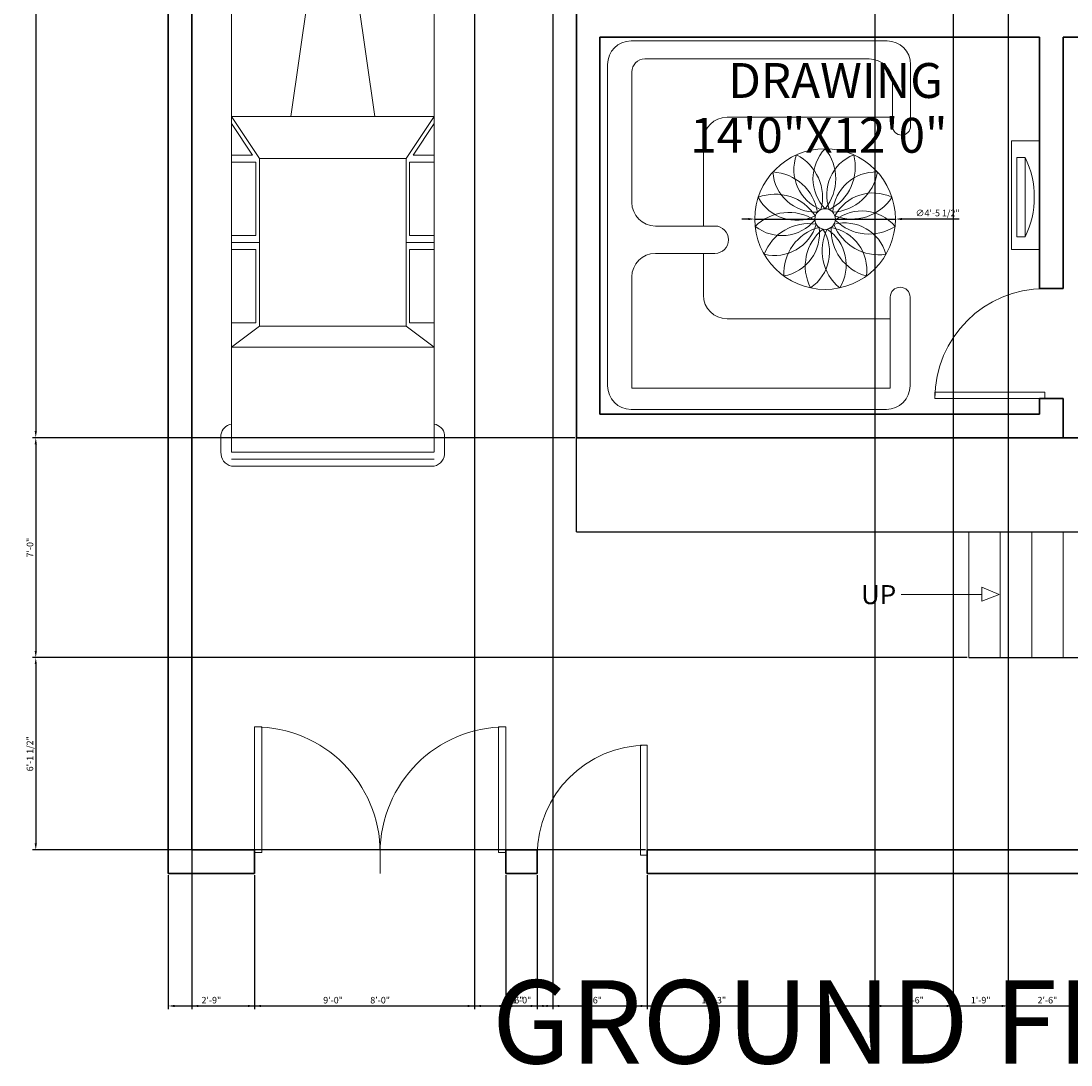
# Model space of a CAD drawing. Units: inches. Extents: x 3412 to 4225, y 13529 to 14581.
# Tile 1 of 7: x 3412 to 3813, y 13529 to 13928. Entities that reach past the tile are written whole.
import ezdxf

# ---------------------------------------------------------------- set-up
doc = ezdxf.new("R2010")
doc.units = ezdxf.units.IN
for name, color, linetype, lineweight in [('A-ANNO-DIMS', 2, 'Continuous', 13), ('A-ANNO-SYMB', 2, 'Continuous', 13), ('A-ANNO-TEXT', 7, 'Continuous', 18), ('A-ANNO-TITL', 7, 'Continuous', 35), ('A-AREA-IDEN', 7, 'Continuous', 18), ('A-DOOR', 4, 'Continuous', 18), ('A-FLOR', 7, 'Continuous', 25), ('A-FLOR-STRS', 3, 'Continuous', 18), ('A-FURN', 8, 'Continuous', 18), ('A-WALL', 7, 'Continuous', 35), ('C-PKNG-VEHI', 8, 'Continuous', 13), ('C-SITE-GATE', 4, 'Continuous', 18), ('C-SITE-WALL', 7, 'Continuous', 35)]:
    doc.layers.add(name, color=color, linetype=linetype, lineweight=lineweight)
doc.styles.get("Standard").update_dxf_attribs({"font": 'arial.ttf'})
doc.dimstyles.new('ISO-25', dxfattribs={"dimtxt": 2.5, "dimasz": 2.5, "dimexe": 1.25, "dimexo": 0.625, "dimtad": 1, "dimdec": 0, "dimlunit": 3, "dimtxsty": 'Standard', "dimcen": 2.5, "dimadec": 0, "dimazin": 0, "dimtfac": 1, "dimtdec": 0, "dimtmove": 0, "dimatfit": 3, "dimfxl": 1, "dimarcsym": 0})

# ---------------------------------------------------------------- blocks, each defined once
blk = doc.blocks.new('*U3')
for p, q in [((0, 0), (0, -5)), ((30, 0), (30, -5))]:
    blk.add_line(p, q)
blk.add_lwpolyline([(0, 0), (0, 30), (1.75, 30), (1.75, 0)], close=True)
blk.add_arc((0, 0), 30, 0, 90)
blk = doc.blocks.new('*U8')
for centre, radius, start, end in [((12.16, 0), 16.5, 135.9523, 224.0477), ((-13.92, 0), 18.27, 321.0981, 38.9019)]:
    blk.add_arc(centre, radius, start, end)
blk = doc.blocks.new('*U9')
at = {"layer": 'A-FURN', "color": 0, "linetype": 'ByBlock', "lineweight": -2, "transparency": 16777216}
for p, rotation in [((3712.86, 13866.4), 24.00000000000002), ((3725.39, 13866.64), 336.0000000000001), ((3707.75, 13862.54), 48.00000000000004), ((3730.64, 13862.98), 312), ((3704.65, 13856.93), 72.00000000000001), ((3733.95, 13857.49), 288), ((3704.11, 13850.55), 96.00000000000003), ((3734.74, 13851.14), 264.0000000000001), ((3706.2, 13844.5), 120), ((3710.58, 13839.82), 144), ((3728.68, 13840.17), 216), ((3732.88, 13845.01), 240), ((3716.48, 13837.33), 168), ((3722.88, 13837.45), 192)]:
    blk.add_blockref('*U8', p, dxfattribs=dict(at, rotation=rotation))
blk.add_blockref('*U8', (3719.1, 13867.85), dxfattribs=at)
blk = doc.blocks.new('*U20')
for p, q in [((5.44, 42.31), (12.12, 42.31)), ((189.69, 42.31), (183.01, 42.31)), ((0.1, -0.41), (0.1, 38.35)), ((2.77, -0.41), (2.77, 38.31)), ((5.44, -0.41), (5.44, 38.24)), ((5.45, 38.31), (16.12, 38.31)), ((16.12, 38.31), (180.34, 38.31)), ((61.52, -0.41), (61.52, 38.31)), ((61.52, 38.31), (77.54, 27.62)), ((64.19, 38.31), (76.2, 30.29)), ((76.2, 30.29), (76.2, 38.31)), ((78.87, 38.31), (78.87, 28.96)), ((106.91, 28.96), (106.91, 38.31)), ((109.58, 27.62), (109.58, 38.31)), ((112.25, 38.31), (112.25, 28.96)), ((140.29, 28.96), (140.29, 38.31)), ((141.62, 27.62), (149.64, 38.31)), ((149.64, -0.41), (149.64, 38.31)), ((189.69, 38.31), (179.01, 38.31)), ((189.69, -0.41), (189.69, 38.24)), ((192.36, -0.41), (192.36, 38.31)), ((195.03, -0.41), (195.03, 38.35)), ((78.87, 28.96), (106.91, 28.96)), ((112.25, 28.96), (140.29, 28.96)), ((77.54, 27.62), (141.62, 27.62)), ((77.54, -0.41), (77.54, 27.62)), ((141.62, -0.41), (141.62, 27.62)), ((5.44, 7.6), (61.52, 15.61)), ((0.1, -0.42), (0.1, -39.18)), ((2.77, -0.41), (2.77, -39.13)), ((5.44, -0.42), (5.44, -39.07)), ((61.52, -0.41), (61.52, -39.13)), ((77.54, -0.41), (77.54, -28.45)), ((141.62, -0.41), (141.62, -28.45)), ((149.64, -0.41), (149.64, -39.13)), ((189.69, -0.42), (189.69, -39.07)), ((192.36, -0.41), (192.36, -39.13)), ((195.03, -0.42), (195.03, -39.18)), ((5.44, -8.42), (61.52, -16.43)), ((61.52, -39.13), (77.54, -28.45)), ((64.19, -39.13), (76.2, -31.12)), ((76.2, -31.12), (76.2, -39.13)), ((77.54, -28.45), (141.62, -28.45)), ((78.87, -39.13), (78.87, -29.79)), ((78.87, -29.79), (106.91, -29.79)), ((106.91, -29.79), (106.91, -39.13)), ((109.58, -28.45), (109.58, -39.13)), ((112.25, -29.79), (140.29, -29.79)), ((112.25, -39.13), (112.25, -29.79)), ((140.29, -29.79), (140.29, -39.13)), ((141.62, -28.45), (149.64, -39.13)), ((5.45, -39.13), (16.12, -39.13)), ((16.12, -39.13), (180.34, -39.13)), ((189.69, -39.13), (179.01, -39.13)), ((5.44, -43.14), (12.12, -43.14)), ((189.69, -43.14), (183.01, -43.14))]:
    blk.add_line(p, q)
for centre, radius, start, end in [((5.06, 37.26), 5.06, 85.6455, 168.0943), ((11.45, 37.64), 4.72, 8.1301, 81.87), ((183.68, 37.64), 4.72, 98.13, 171.8699), ((190.07, 37.26), 5.06, 11.9057, 94.3545), ((5.06, -38.09), 5.06, 191.9057, 274.3545), ((11.45, -38.46), 4.72, 278.13, 351.8699), ((183.68, -38.46), 4.72, 188.1301, 261.87), ((190.07, -38.09), 5.06, 265.6455, 348.0943)]:
    blk.add_arc(centre, radius, start, end)
blk = doc.blocks.new('ARROW-ENTRY-STEP')
for p, q in [((30.86, 5.34), (37.49, 2.66)), ((30.86, 0), (30.86, 5.34)), ((0, 2.66), (30.86, 2.66)), ((37.49, 2.66), (30.86, 0))]:
    blk.add_line(p, q)
blk = doc.blocks.new('ENTRY-STEP-FLIGHT')
for p, q in [((0, 48), (0, 0)), ((12, 48), (12, 0)), ((24, 48), (24, 0)), ((36, 48), (36, 0))]:
    blk.add_line(p, q)
blk = doc.blocks.new('*D61')
at = {"layer": 'A-ANNO-DIMS', "color": 0, "lineweight": -2, "transparency": 16777216}
for p, q in [((3477.36, 14408.81), (3477.36, 13550.58)), ((3585.36, 14408.81), (3585.36, 13550.58)), ((3479.86, 13551.83), (3582.86, 13551.83))]:
    blk.add_line(p, q, dxfattribs=at)
at = {"layer": 'A-ANNO-DIMS', "color": 0, "transparency": 16777216}
for points in [[(3479.86, 13552.25), (3479.86, 13551.42), (3477.36, 13551.83)], [(3582.86, 13552.25), (3582.86, 13551.42), (3585.36, 13551.83)]]:
    blk.add_solid(points, dxfattribs=at)
at = {"layer": 'Defpoints', "color": 0, "transparency": 16777216}
for p in [(3477.36, 14409.43), (3585.36, 14409.43), (3585.36, 13551.83)]:
    blk.add_point(p, dxfattribs=at)
at = {"layer": 'A-ANNO-DIMS', "color": 0, "transparency": 16777216, "insert": (3531.36, 13553.73), "char_height": 2.5, "attachment_point": 5}
blk.add_mtext('9\'-0"', dxfattribs=at)
blk = doc.blocks.new('*D62')
at = {"layer": 'A-ANNO-DIMS', "color": 0, "lineweight": -2, "transparency": 16777216}
for p, q in [((3585.36, 14408.81), (3585.36, 13550.58)), ((3615.36, 14408.81), (3615.36, 13550.58)), ((3587.86, 13551.83), (3612.86, 13551.83))]:
    blk.add_line(p, q, dxfattribs=at)
at = {"layer": 'A-ANNO-DIMS', "color": 0, "transparency": 16777216}
for points in [[(3587.86, 13552.25), (3587.86, 13551.42), (3585.36, 13551.83)], [(3612.86, 13552.25), (3612.86, 13551.42), (3615.36, 13551.83)]]:
    blk.add_solid(points, dxfattribs=at)
at = {"layer": 'Defpoints', "color": 0, "transparency": 16777216}
for p in [(3585.36, 14409.43), (3615.36, 14409.43), (3615.36, 13551.83)]:
    blk.add_point(p, dxfattribs=at)
at = {"layer": 'A-ANNO-DIMS', "color": 0, "transparency": 16777216, "insert": (3600.36, 13553.73), "char_height": 2.5, "attachment_point": 5}
blk.add_mtext('2\'-6"', dxfattribs=at)
blk = doc.blocks.new('*D63')
at = {"layer": 'A-ANNO-DIMS', "color": 0, "lineweight": -2, "transparency": 16777216}
for p, q in [((3615.36, 14408.81), (3615.36, 13550.58)), ((3738.36, 14408.81), (3738.36, 13550.58)), ((3617.86, 13551.83), (3735.86, 13551.83))]:
    blk.add_line(p, q, dxfattribs=at)
at = {"layer": 'A-ANNO-DIMS', "color": 0, "transparency": 16777216}
for points in [[(3617.86, 13552.25), (3617.86, 13551.42), (3615.36, 13551.83)], [(3735.86, 13552.25), (3735.86, 13551.42), (3738.36, 13551.83)]]:
    blk.add_solid(points, dxfattribs=at)
at = {"layer": 'Defpoints', "color": 0, "transparency": 16777216}
for p in [(3615.36, 14409.43), (3738.36, 14409.43), (3738.36, 13551.83)]:
    blk.add_point(p, dxfattribs=at)
at = {"layer": 'A-ANNO-DIMS', "color": 0, "transparency": 16777216, "insert": (3676.86, 13553.73), "char_height": 2.5, "attachment_point": 5}
blk.add_mtext('10\'-3"', dxfattribs=at)
blk = doc.blocks.new('*D64')
at = {"layer": 'A-ANNO-DIMS', "color": 0, "lineweight": -2, "transparency": 16777216}
for p, q in [((3738.36, 14408.81), (3738.36, 13550.58)), ((3768.36, 14408.81), (3768.36, 13550.58)), ((3740.86, 13551.83), (3765.86, 13551.83))]:
    blk.add_line(p, q, dxfattribs=at)
at = {"layer": 'A-ANNO-DIMS', "color": 0, "transparency": 16777216}
for points in [[(3740.86, 13552.25), (3740.86, 13551.42), (3738.36, 13551.83)], [(3765.86, 13552.25), (3765.86, 13551.42), (3768.36, 13551.83)]]:
    blk.add_solid(points, dxfattribs=at)
at = {"layer": 'Defpoints', "color": 0, "transparency": 16777216}
for p in [(3738.36, 14409.43), (3768.36, 14409.43), (3768.36, 13551.83)]:
    blk.add_point(p, dxfattribs=at)
at = {"layer": 'A-ANNO-DIMS', "color": 0, "transparency": 16777216, "insert": (3753.36, 13553.73), "char_height": 2.5, "attachment_point": 5}
blk.add_mtext('2\'-6"', dxfattribs=at)
blk = doc.blocks.new('*D65')
at = {"layer": 'A-ANNO-DIMS', "color": 0, "lineweight": -2, "transparency": 16777216}
for p, q in [((3768.36, 14408.81), (3768.36, 13550.58)), ((3789.36, 14408.81), (3789.36, 13550.58)), ((3770.86, 13551.83), (3786.86, 13551.83))]:
    blk.add_line(p, q, dxfattribs=at)
at = {"layer": 'A-ANNO-DIMS', "color": 0, "transparency": 16777216}
for points in [[(3770.86, 13552.25), (3770.86, 13551.42), (3768.36, 13551.83)], [(3786.86, 13552.25), (3786.86, 13551.42), (3789.36, 13551.83)]]:
    blk.add_solid(points, dxfattribs=at)
at = {"layer": 'Defpoints', "color": 0, "transparency": 16777216}
for p in [(3768.36, 14409.43), (3789.36, 14409.43), (3789.36, 13551.83)]:
    blk.add_point(p, dxfattribs=at)
at = {"layer": 'A-ANNO-DIMS', "color": 0, "transparency": 16777216, "insert": (3778.86, 13553.73), "char_height": 2.5, "attachment_point": 5}
blk.add_mtext('1\'-9"', dxfattribs=at)
blk = doc.blocks.new('*D66')
at = {"layer": 'A-ANNO-DIMS', "color": 0, "lineweight": -2, "transparency": 16777216}
for p, q in [((3789.36, 14408.81), (3789.36, 13550.58)), ((3819.36, 14408.81), (3819.36, 13550.58)), ((3791.86, 13551.83), (3816.86, 13551.83))]:
    blk.add_line(p, q, dxfattribs=at)
at = {"layer": 'A-ANNO-DIMS', "color": 0, "transparency": 16777216}
for points in [[(3791.86, 13552.25), (3791.86, 13551.42), (3789.36, 13551.83)], [(3816.86, 13552.25), (3816.86, 13551.42), (3819.36, 13551.83)]]:
    blk.add_solid(points, dxfattribs=at)
at = {"layer": 'Defpoints', "color": 0, "transparency": 16777216}
for p in [(3789.36, 14409.43), (3819.36, 14409.43), (3819.36, 13551.83)]:
    blk.add_point(p, dxfattribs=at)
at = {"layer": 'A-ANNO-DIMS', "color": 0, "transparency": 16777216, "insert": (3804.36, 13553.73), "char_height": 2.5, "attachment_point": 5}
blk.add_mtext('2\'-6"', dxfattribs=at)
blk = doc.blocks.new('*D74')
at = {"layer": 'A-ANNO-DIMS', "color": 0, "lineweight": -2, "transparency": 16777216}
for p, q in [((3593.73, 14199.43), (3416.51, 14199.43)), ((3417.76, 14196.93), (3417.76, 13771.43)), ((3623.73, 13768.93), (3416.51, 13768.93))]:
    blk.add_line(p, q, dxfattribs=at)
at = {"layer": 'A-ANNO-DIMS', "color": 0, "transparency": 16777216}
for points in [[(3417.34, 14196.93), (3418.17, 14196.93), (3417.76, 14199.43)], [(3417.34, 13771.43), (3418.17, 13771.43), (3417.76, 13768.93)]]:
    blk.add_solid(points, dxfattribs=at)
at = {"layer": 'Defpoints', "color": 0, "transparency": 16777216}
for p in [(3594.36, 14199.43), (3417.76, 13768.93), (3624.36, 13768.93)]:
    blk.add_point(p, dxfattribs=at)
at = {"layer": 'A-ANNO-DIMS', "color": 0, "transparency": 16777216, "insert": (3415.84, 13984.18), "char_height": 2.5, "attachment_point": 5, "rotation": 90}
blk.add_mtext('35\'-10 1/2"', dxfattribs=at)
blk = doc.blocks.new('*D75')
at = {"layer": 'A-ANNO-DIMS', "color": 0, "lineweight": -2, "transparency": 16777216}
for p, q in [((3623.73, 13768.93), (3416.51, 13768.93)), ((3417.76, 13766.43), (3417.76, 13687.43)), ((3773.73, 13684.93), (3416.51, 13684.93))]:
    blk.add_line(p, q, dxfattribs=at)
at = {"layer": 'A-ANNO-DIMS', "color": 0, "transparency": 16777216}
for points in [[(3417.34, 13766.43), (3418.17, 13766.43), (3417.76, 13768.93)], [(3417.34, 13687.43), (3418.17, 13687.43), (3417.76, 13684.93)]]:
    blk.add_solid(points, dxfattribs=at)
at = {"layer": 'Defpoints', "color": 0, "transparency": 16777216}
for p in [(3624.36, 13768.93), (3417.76, 13684.93), (3774.36, 13684.93)]:
    blk.add_point(p, dxfattribs=at)
at = {"layer": 'A-ANNO-DIMS', "color": 0, "transparency": 16777216, "insert": (3415.86, 13726.93), "char_height": 2.5, "attachment_point": 5, "rotation": 90}
blk.add_mtext('7\'-0"', dxfattribs=at)
blk = doc.blocks.new('*D76')
at = {"layer": 'A-ANNO-DIMS', "color": 0, "lineweight": -2, "transparency": 16777216}
for p, q in [((3773.73, 13684.93), (3416.51, 13684.93)), ((3417.76, 13682.43), (3417.76, 13613.93)), ((3650.73, 13611.43), (3416.51, 13611.43))]:
    blk.add_line(p, q, dxfattribs=at)
at = {"layer": 'A-ANNO-DIMS', "color": 0, "transparency": 16777216}
for points in [[(3417.34, 13682.43), (3418.17, 13682.43), (3417.76, 13684.93)], [(3417.34, 13613.93), (3418.17, 13613.93), (3417.76, 13611.43)]]:
    blk.add_solid(points, dxfattribs=at)
at = {"layer": 'Defpoints', "color": 0, "transparency": 16777216}
for p in [(3774.36, 13684.93), (3417.76, 13611.43), (3651.36, 13611.43)]:
    blk.add_point(p, dxfattribs=at)
at = {"layer": 'A-ANNO-DIMS', "color": 0, "transparency": 16777216, "insert": (3415.84, 13648.18), "char_height": 2.5, "attachment_point": 5, "rotation": 90}
blk.add_mtext('6\'-1 1/2"', dxfattribs=at)
blk = doc.blocks.new('*D77')
at = {"layer": 'A-ANNO-DIMS', "color": 0, "lineweight": -2, "transparency": 16777216}
for p, q in [((3468.36, 13601.81), (3468.36, 13550.58)), ((3501.36, 13601.81), (3501.36, 13550.58)), ((3470.86, 13551.83), (3498.86, 13551.83))]:
    blk.add_line(p, q, dxfattribs=at)
at = {"layer": 'A-ANNO-DIMS', "color": 0, "transparency": 16777216}
for points in [[(3470.86, 13552.25), (3470.86, 13551.42), (3468.36, 13551.83)], [(3498.86, 13552.25), (3498.86, 13551.42), (3501.36, 13551.83)]]:
    blk.add_solid(points, dxfattribs=at)
at = {"layer": 'Defpoints', "color": 0, "transparency": 16777216}
for p in [(3468.36, 13602.43), (3501.36, 13602.43), (3501.36, 13551.83)]:
    blk.add_point(p, dxfattribs=at)
at = {"layer": 'A-ANNO-DIMS', "color": 0, "transparency": 16777216, "insert": (3484.86, 13553.73), "char_height": 2.5, "attachment_point": 5}
blk.add_mtext('2\'-9"', dxfattribs=at)
blk = doc.blocks.new('*D78')
at = {"layer": 'A-ANNO-DIMS', "color": 0, "lineweight": -2, "transparency": 16777216}
for p, q in [((3501.36, 13601.81), (3501.36, 13550.58)), ((3597.36, 13601.81), (3597.36, 13550.58)), ((3503.86, 13551.83), (3594.86, 13551.83))]:
    blk.add_line(p, q, dxfattribs=at)
at = {"layer": 'A-ANNO-DIMS', "color": 0, "transparency": 16777216}
for points in [[(3503.86, 13552.25), (3503.86, 13551.42), (3501.36, 13551.83)], [(3594.86, 13552.25), (3594.86, 13551.42), (3597.36, 13551.83)]]:
    blk.add_solid(points, dxfattribs=at)
at = {"layer": 'Defpoints', "color": 0, "transparency": 16777216}
for p in [(3501.36, 13602.43), (3597.36, 13602.43), (3597.36, 13551.83)]:
    blk.add_point(p, dxfattribs=at)
at = {"layer": 'A-ANNO-DIMS', "color": 0, "transparency": 16777216, "insert": (3549.36, 13553.73), "char_height": 2.5, "attachment_point": 5}
blk.add_mtext('8\'-0"', dxfattribs=at)
blk = doc.blocks.new('*D79')
at = {"layer": 'A-ANNO-DIMS', "color": 0, "lineweight": -2, "transparency": 16777216}
for p, q in [((3597.36, 13601.81), (3597.36, 13550.58)), ((3609.36, 13601.81), (3609.36, 13550.58)), ((3599.86, 13551.83), (3606.86, 13551.83))]:
    blk.add_line(p, q, dxfattribs=at)
at = {"layer": 'A-ANNO-DIMS', "color": 0, "transparency": 16777216}
for points in [[(3599.86, 13552.25), (3599.86, 13551.42), (3597.36, 13551.83)], [(3606.86, 13552.25), (3606.86, 13551.42), (3609.36, 13551.83)]]:
    blk.add_solid(points, dxfattribs=at)
at = {"layer": 'Defpoints', "color": 0, "transparency": 16777216}
for p in [(3597.36, 13602.43), (3609.36, 13602.43), (3609.36, 13551.83)]:
    blk.add_point(p, dxfattribs=at)
at = {"layer": 'A-ANNO-DIMS', "color": 0, "transparency": 16777216, "insert": (3603.36, 13553.73), "char_height": 2.5, "attachment_point": 5}
blk.add_mtext('1\'-0"', dxfattribs=at)
blk = doc.blocks.new('*D80')
at = {"layer": 'A-ANNO-DIMS', "color": 0, "lineweight": -2, "transparency": 16777216}
for p, q in [((3609.36, 13601.81), (3609.36, 13550.58)), ((3651.36, 13601.81), (3651.36, 13550.58)), ((3611.86, 13551.83), (3648.86, 13551.83))]:
    blk.add_line(p, q, dxfattribs=at)
at = {"layer": 'A-ANNO-DIMS', "color": 0, "transparency": 16777216}
for points in [[(3611.86, 13552.25), (3611.86, 13551.42), (3609.36, 13551.83)], [(3648.86, 13552.25), (3648.86, 13551.42), (3651.36, 13551.83)]]:
    blk.add_solid(points, dxfattribs=at)
at = {"layer": 'Defpoints', "color": 0, "transparency": 16777216}
for p in [(3609.36, 13602.43), (3651.36, 13602.43), (3651.36, 13551.83)]:
    blk.add_point(p, dxfattribs=at)
at = {"layer": 'A-ANNO-DIMS', "color": 0, "transparency": 16777216, "insert": (3630.36, 13553.73), "char_height": 2.5, "attachment_point": 5}
blk.add_mtext('3\'-6"', dxfattribs=at)
blk = doc.blocks.new('*D86')
at = {"layer": 'A-ANNO-DIMS', "color": 0, "lineweight": -2, "transparency": 16777216}
for p, q in [((3690.02, 13852.45), (3687.52, 13852.45)), ((3692.52, 13852.45), (3746.27, 13852.45)), ((3770.61, 13852.45), (3748.77, 13852.45))]:
    blk.add_line(p, q, dxfattribs=at)
at = {"layer": 'A-ANNO-DIMS', "color": 0, "transparency": 16777216}
for points in [[(3690.02, 13852.87), (3690.02, 13852.04), (3692.52, 13852.45)], [(3748.77, 13852.87), (3748.77, 13852.04), (3746.27, 13852.45)]]:
    blk.add_solid(points, dxfattribs=at)
at = {"layer": 'Defpoints', "color": 0, "transparency": 16777216}
for p in [(3692.52, 13852.45), (3746.27, 13852.45)]:
    blk.add_point(p, dxfattribs=at)
at = {"layer": 'A-ANNO-DIMS', "color": 0, "transparency": 16777216, "insert": (3762.39, 13854.43), "char_height": 2.5, "attachment_point": 5, "rotation": 359.9996}
blk.add_mtext('∅4\'-5 1/2"', dxfattribs=at)

msp = doc.modelspace()

# ---------------------------------------------------------------- linework, layer by layer
at = {"layer": 'A-FLOR'}
for p, q in [((3624.36, 13732.93), (3624.36, 13768.93)), ((3624.36, 13732.93), (3843.36, 13732.93)), ((3774.36, 13684.93), (3984.36, 13684.93))]:
    msp.add_line(p, q, dxfattribs=at)
at = {"layer": 'A-FURN'}
for p, q in [((3743.08, 13920.53), (3645.25, 13920.53)), ((3736.19, 13913.64), (3650.54, 13913.64)), ((3636.25, 13911.53), (3636.25, 13788.75)), ((3645.54, 13908.64), (3645.54, 13858.8)), ((3752.08, 13887.99), (3752.08, 13911.53)), ((3745.19, 13904.64), (3745.19, 13887.99)), ((3745.19, 13891.37), (3681.91, 13891.37)), ((3672.91, 13882.37), (3672.91, 13849.8)), ((3654.54, 13849.8), (3677.29, 13849.8)), ((3677.29, 13839.34), (3654.54, 13839.34)), ((3672.91, 13839.34), (3672.91, 13823.38)), ((3645.54, 13787.85), (3645.54, 13830.34)), ((3744.29, 13787.85), (3744.29, 13822.63)), ((3751.86, 13822.63), (3751.86, 13788.75)), ((3681.91, 13814.38), (3744.29, 13814.38)), ((3645.54, 13787.85), (3744.29, 13787.85)), ((3742.86, 13779.75), (3645.25, 13779.75))]:
    msp.add_line(p, q, dxfattribs=at)
for points in [[(3801.36, 13882.34), (3790.59, 13882.34), (3790.59, 13840.88), (3801.36, 13840.88)], [(3792.63, 13875.99), (3795.84, 13875.99), (3795.84, 13845.68), (3792.63, 13845.68)]]:
    msp.add_lwpolyline(points, close=True, dxfattribs=at)
for radius in [26.87, 3.93]:
    msp.add_circle((3719.39, 13852.45), radius, dxfattribs=at)
for centre, radius, start, end in [((3645.25, 13911.53), 9, 90, 180), ((3743.08, 13911.53), 9, 0, 90), ((3650.54, 13908.64), 5, 90, 180), ((3736.19, 13904.64), 9, 0, 90), ((3681.91, 13882.37), 9, 90, 180), ((3748.63, 13887.99), 3.44, 180, 0), ((3764.77, 13860.83), 34.57, 334.0016, 25.9984), ((3654.54, 13858.8), 9, 180, 270), ((3677.29, 13844.57), 5.23, 270, 90), ((3654.54, 13830.34), 9, 90, 180), ((3681.91, 13823.38), 9, 180, 270), ((3748.08, 13822.63), 3.78, 0, 180), ((3645.25, 13788.75), 9, 180, 270), ((3742.86, 13788.75), 9, 270, 0)]:
    msp.add_arc(centre, radius, start, end, dxfattribs=at)
at = {"layer": 'A-WALL'}
for p, q in [((3624.36, 14007.43), (3624.36, 13768.93)), ((3633.36, 13921.93), (3801.36, 13921.93)), ((3633.36, 13921.93), (3633.36, 13777.93)), ((3801.36, 13921.93), (3801.36, 13825.93)), ((3810.36, 13921.93), (3810.36, 13825.93)), ((3810.36, 13921.93), (3855.36, 13921.93)), ((3801.36, 13825.93), (3810.36, 13825.93)), ((3801.36, 13783.93), (3810.36, 13783.93)), ((3801.36, 13783.93), (3801.36, 13777.93)), ((3810.36, 13783.93), (3810.36, 13777.93)), ((3810.36, 13783.93), (3810.36, 13768.93)), ((3633.36, 13777.93), (3801.36, 13777.93)), ((3624.36, 13768.93), (3843.36, 13768.93))]:
    msp.add_line(p, q, dxfattribs=at)
at = {"layer": 'C-SITE-WALL'}
for p, q in [((3468.36, 14526.43), (3468.36, 13602.43)), ((3477.36, 14409.43), (3477.36, 13611.43)), ((3477.36, 13611.43), (3501.36, 13611.43)), ((3501.36, 13611.43), (3501.36, 13602.43)), ((3597.36, 13611.43), (3597.36, 13602.43)), ((3597.36, 13611.43), (3609.36, 13611.43)), ((3609.36, 13611.43), (3609.36, 13602.43)), ((3651.36, 13611.43), (3651.36, 13602.43)), ((3651.36, 13611.43), (4044.36, 13611.43)), ((3468.36, 13602.43), (3501.36, 13602.43)), ((3597.36, 13602.43), (3609.36, 13602.43)), ((3651.36, 13602.43), (4044.36, 13602.43))]:
    msp.add_line(p, q, dxfattribs=at)

# ---------------------------------------------------------------- block references
at = {"layer": 'A-ANNO-SYMB'}
msp.add_blockref('ARROW-ENTRY-STEP', (3748.46, 13706.43), dxfattribs=at)
at = {"layer": 'A-DOOR', "xscale": 1.399999999999999, "yscale": 1.399999999999999, "zscale": 1.399999999999999, "rotation": 89.99999999999999}
msp.add_blockref('*U3', (3803.36, 13783.93), dxfattribs=at)
at = {"layer": 'A-FLOR-STRS', "extrusion": (0, 0, -1), "zscale": -1}
msp.add_blockref('ENTRY-STEP-FLIGHT', (-3810.36, 13684.93), dxfattribs=at)
at = {"layer": 'A-FURN'}
msp.add_blockref('*U9', (0, 0), dxfattribs=at)
at = {"layer": 'C-PKNG-VEHI', "rotation": 270}
msp.add_blockref('*U20', (3531.67, 13953.1), dxfattribs=at)
at = {"layer": 'C-SITE-GATE'}
for p, xscale, yscale, zscale in [((3501.36, 13610.43), 1.599999999999999, 1.599999999999999, 1.599999999999999), ((3597.36, 13610.43), -1.599999999999999, 1.599999999999999, 1.599999999999999), ((3651.36, 13609.43), -1.399999999999999, 1.399999999999999, 1.399999999999999)]:
    msp.add_blockref('*U3', p, dxfattribs=dict(at, xscale=xscale, yscale=yscale, zscale=zscale))

# ---------------------------------------------------------------- texts
at = {"layer": 'A-ANNO-TEXT'}
msp.add_text('UP', height=7.282, dxfattribs=at).set_placement((3733.12, 13705.34))
at = {"layer": 'A-ANNO-TITL'}
msp.add_text('GROUND FLOOR PLAN', height=31.8222, dxfattribs=at).set_placement((3592.1, 13529.85))
at = {"layer": 'A-AREA-IDEN'}
for s, height, p in [('DRAWING', 13.329, (3682.37, 13898.72)), ('14\'0"X12\'0"', 13.3293, (3667.87, 13877.79))]:
    msp.add_text(s, height=height, dxfattribs=at).set_placement(p)

# ---------------------------------------------------------------- dimensions: what is measured, and where the dimension line sits
at = {"layer": 'A-ANNO-DIMS'}
for base, p1, p2, picture, middle in [((3585.36, 13551.83), (3477.36, 14409.43), (3585.36, 14409.43), '*D61', (3531.36, 13553.73)), ((3615.36, 13551.83), (3585.36, 14409.43), (3615.36, 14409.43), '*D62', (3600.36, 13553.73)), ((3738.36, 13551.83), (3615.36, 14409.43), (3738.36, 14409.43), '*D63', (3676.86, 13553.73)), ((3768.36, 13551.83), (3738.36, 14409.43), (3768.36, 14409.43), '*D64', (3753.36, 13553.73)), ((3789.36, 13551.83), (3768.36, 14409.43), (3789.36, 14409.43), '*D65', (3778.86, 13553.73)), ((3819.36, 13551.83), (3789.36, 14409.43), (3819.36, 14409.43), '*D66', (3804.36, 13553.73)), ((3501.36, 13551.83), (3468.36, 13602.43), (3501.36, 13602.43), '*D77', (3484.86, 13553.73)), ((3597.36, 13551.83), (3501.36, 13602.43), (3597.36, 13602.43), '*D78', (3549.36, 13553.73)), ((3609.36, 13551.83), (3597.36, 13602.43), (3609.36, 13602.43), '*D79', (3603.36, 13553.73)), ((3651.36, 13551.83), (3609.36, 13602.43), (3651.36, 13602.43), '*D80', (3630.36, 13553.73))]:
    dim = msp.add_linear_dim(base=base, p1=p1, p2=p2, dimstyle='ISO-25', override={"dimdec": 1, "dimlfac": 1, "dimrnd": 0, "dimzin": 1, "dimdsep": 46, "dimlunit": 4, "dimfrac": 2}, dxfattribs=at)
    dim.commit()
    dim.dimension.update_dxf_attribs({"geometry": picture, "text_midpoint": middle})
for base, p1, p2, picture, middle in [((3417.76, 13768.93), (3594.36, 14199.43), (3624.36, 13768.93), '*D74', (3415.84, 13984.18)), ((3417.76, 13684.93), (3624.36, 13768.93), (3774.36, 13684.93), '*D75', (3415.86, 13726.93)), ((3417.76, 13611.43), (3774.36, 13684.93), (3651.36, 13611.43), '*D76', (3415.84, 13648.18))]:
    dim = msp.add_linear_dim(base=base, p1=p1, p2=p2, angle=90, dimstyle='ISO-25', override={"dimdec": 1, "dimlfac": 1, "dimrnd": 0, "dimzin": 1, "dimdsep": 46, "dimlunit": 4, "dimfrac": 2}, dxfattribs=at)
    dim.commit()
    dim.dimension.update_dxf_attribs({"geometry": picture, "text_midpoint": middle})
dim = msp.add_diameter_dim_2p(p1=(3692.5167, 13852.4544), p2=(3746.2651, 13852.454), dimstyle='ISO-25', override={"dimdec": 1, "dimlfac": 1, "dimrnd": 0, "dimzin": 1, "dimdsep": 46, "dimlunit": 4, "dimfrac": 2}, dxfattribs=at)
dim.commit()
dim.dimension.update_dxf_attribs({"geometry": '*D86', "text_midpoint": (3762.3896, 13852.4539), "dimtype": 163})

doc.saveas('drawing.dxf')
